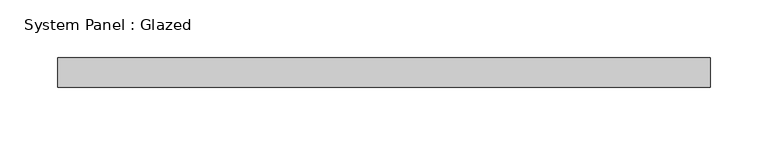
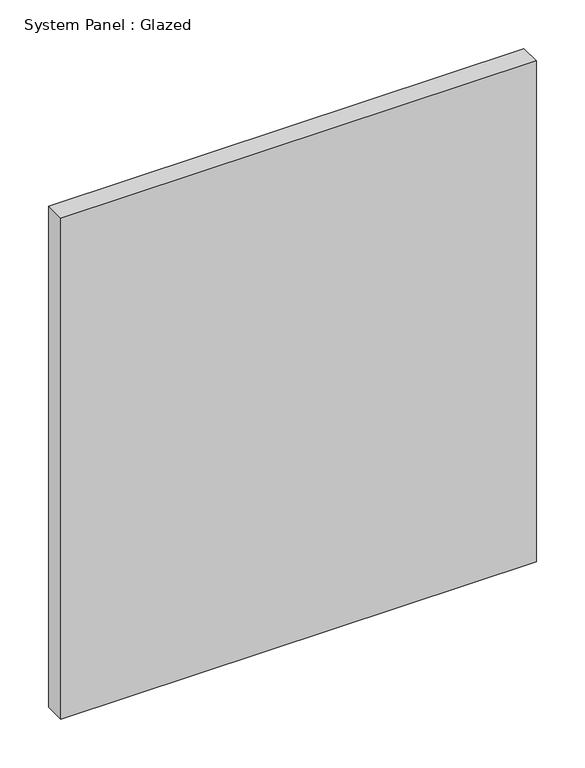
"""IFC4 building model written with IfcOpenShell, lengths in millimetres: plate geometry, System Panel : Glazed."""

from ifc_helpers import new_model, si_unit, origin, origin_with_axes, place, context, project, spatial, polyline, outline, extrude, source, transform, mapped, element, save


def system_panel_glazed_9f6ea25c(model_context):
    return source(origin(), model_context, "Body", "SweptSolid", [
        extrude(outline(polyline([(282.575, 19.05), (-282.575, 19.05), (-282.575, 44.45), (282.575, 44.45), (282.575, 19.05)])), origin_with_axes(), (0.0, 0.0, 1.0), 629.4801773),
    ])


if __name__ == "__main__":
    model = new_model("IFC4")
    model_context = context("Model", 3, world=origin())
    ifc_project = project(units=[si_unit("LENGTHUNIT", "METRE", prefix="MILLI")], contexts=[model_context])
    site = spatial("IfcSite", under=ifc_project)
    building = spatial("IfcBuilding", under=site)
    placement = place(None, origin())
    system_panel_glazed_shape = system_panel_glazed_9f6ea25c(model_context)
    element("IfcPlate", 1, ObjectType="System Panel : Glazed", at=placement, inside=building, context=model_context, shape_type="MappedRepresentation", body=[
        mapped(system_panel_glazed_shape, transform((0.0, 0.0, 0.0), x_axis=(1.0, 0.0, 0.0), y_axis=(0.0, 1.0, 0.0), z_axis=(0.0, 0.0, 1.0))),
    ])
    save(model, "model.ifc")

# Revit data of these elements
# Type "System Panel : Glazed"
#   Construction Type Id = "GSP4R"
#   Analytic Construction = "1/8 in Pilkington single glazing"
#   Visual Light Transmittance = 0.9
#   Solar Heat Gain Coefficient = 0.86
#   Heat Transfer Coefficient (U) = 1.18115 BTU/(h·ft²·°F)
#   Define Thermal Properties by = 1
# Element 1 (IfcPlate, "System Panel : Glazed")
#   Materials on its faces: "Glass"
# Materials
#   "Glass": class "Glass", colour RGB 0 128 192, transparency 0.75, Description = "Soda Lime Glass", Cost = 0
